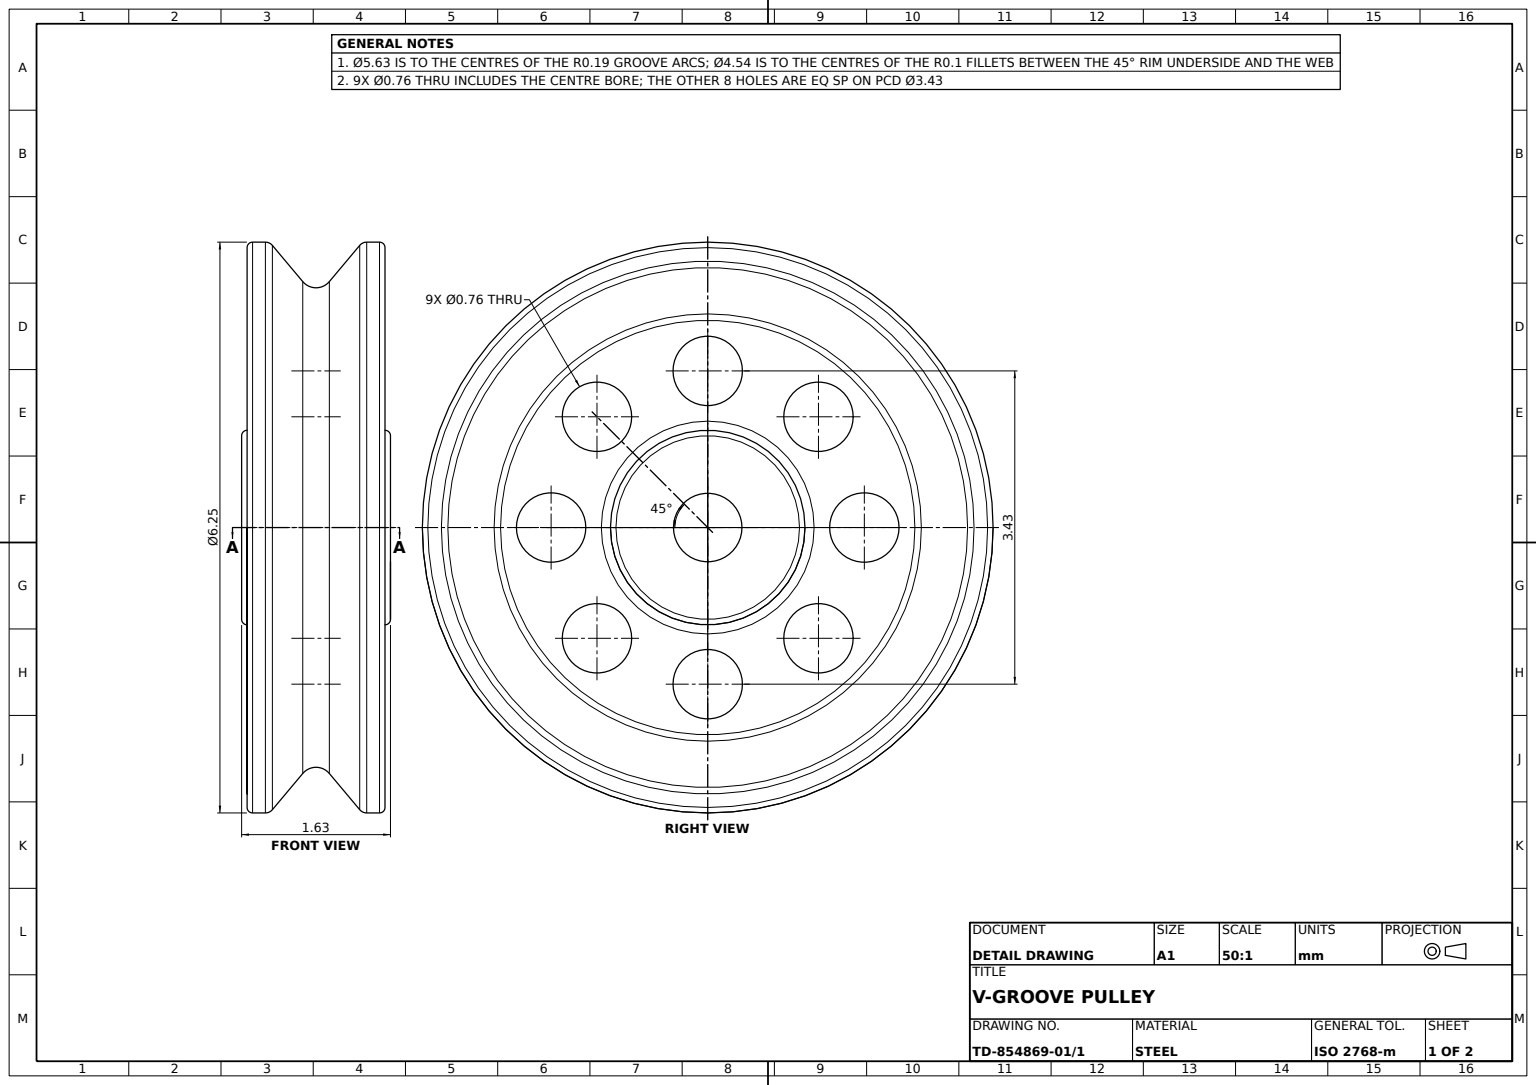
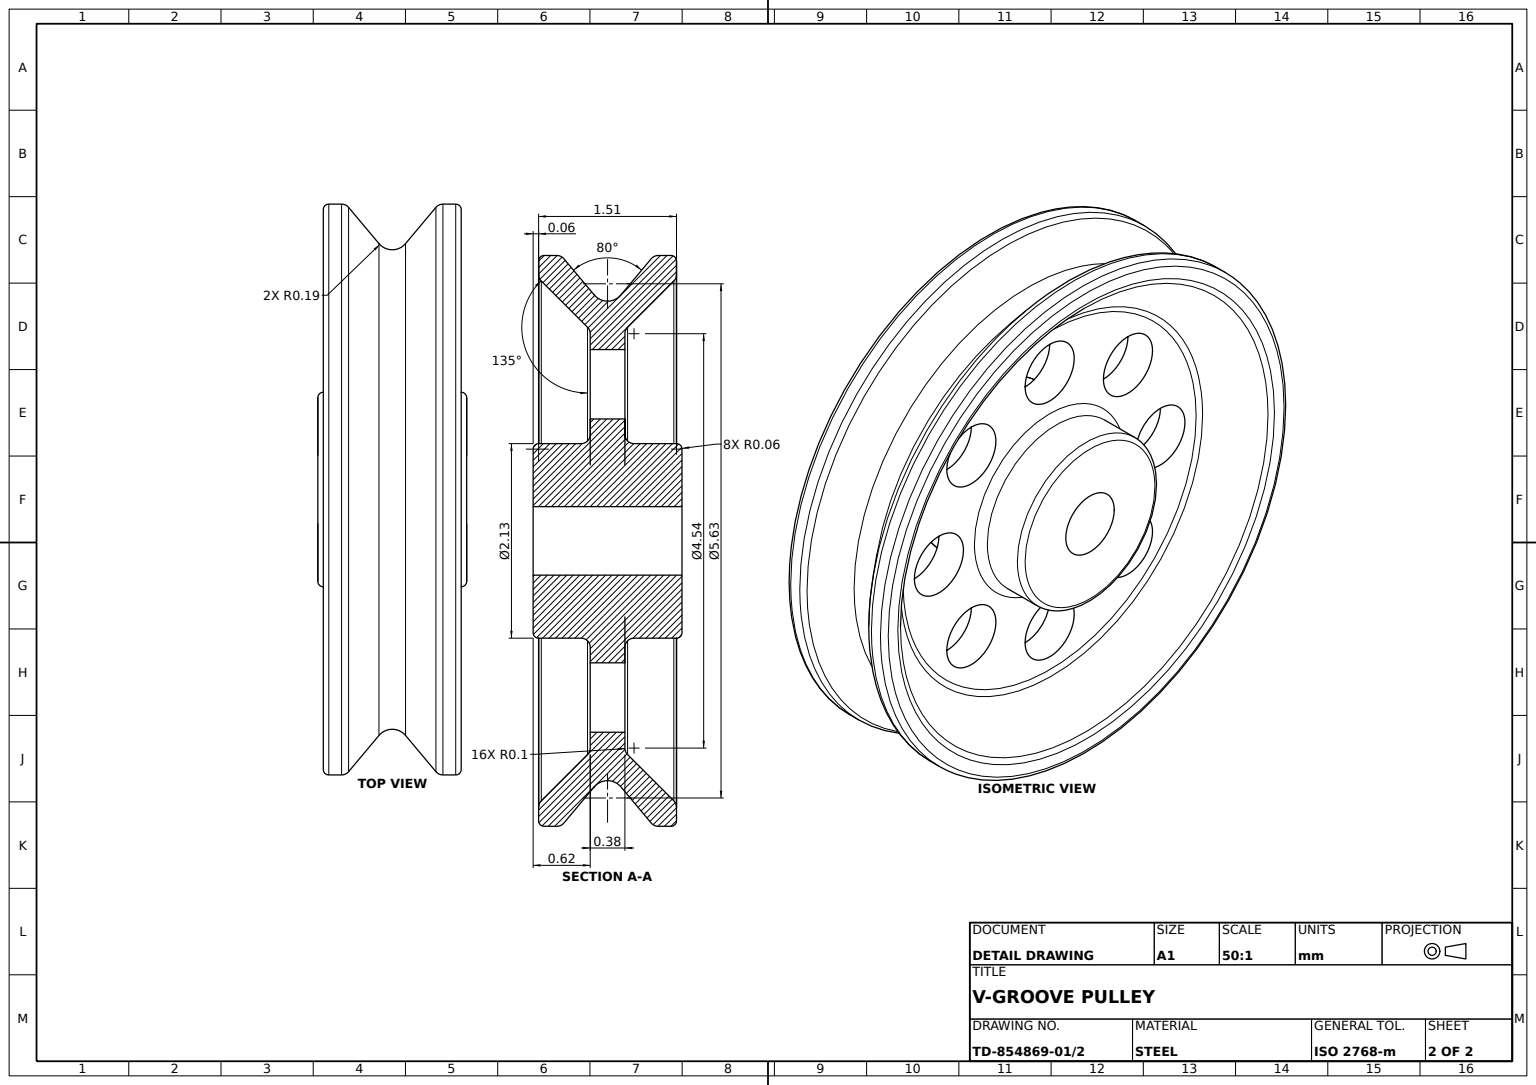
SolidWorks part; units mm, degrees
material "Plain Carbon Steel"
ref_plane "Front Plane" through (0, 0, 0) normal (0, 0, 1) x (1, 0, 0)
ref_plane "Top Plane" through (0, 0, 0) normal (0, 1, 0) x (1, 0, 0)
ref_plane "Right Plane" through (0, 0, 0) normal (1, 0, 0) x (0, 0, -1)
sketch "Pulley Profile Sketch" plane through (0, 0, 0) normal (1, 0, 0) x (0, 0, -1)
  line L0 (-29.196, 0) -> (1430.6033, 0) construction
  line L1 (0, -29.196) -> (0, 1430.6033) construction
  line L2 (0.815, 0.375) -> (-0.815, 0.375)
  line L3 (-0.815, 0.375) -> (-0.815, 1.005)
  line L4 (-0.755, 1.065) -> (-0.29, 1.065)
  line L5 (-0.19, 1.165) -> (-0.19, 2.2686)
  line L6 (-0.2193, 2.3393) -> (-0.7257, 2.8457)
  line L7 (-0.755, 2.9164) -> (-0.755, 3.065)
  line L8 (-0.695, 3.125) -> (-0.5548, 3.125)
  line L9 (-0.4782, 3.0893) -> (-0.1455, 2.6929)
  line L10 (0.1455, 2.6929) -> (0.4782, 3.0893)
  line L11 (0.5548, 3.125) -> (0.695, 3.125)
  line L12 (0.755, 3.065) -> (0.755, 2.9164)
  line L13 (0.7257, 2.8457) -> (0.2193, 2.3393)
  line L14 (0.19, 2.2686) -> (0.19, 1.165)
  line L15 (0.29, 1.065) -> (0.755, 1.065)
  line L16 (0.815, 1.005) -> (0.815, 0.375)
  arc A0 (-0.1455, 2.6929) -> (0.1455, 2.6929) centre (0, 2.815) ccw
  arc A1 (-0.755, 2.9164) -> (-0.7257, 2.8457) centre (-0.655, 2.9164) ccw
  arc A2 (0.755, 2.9164) -> (0.7257, 2.8457) centre (0.655, 2.9164) cw
  arc A3 (0.5548, 3.125) -> (0.4782, 3.0893) centre (0.5548, 3.025) ccw
  arc A4 (-0.4782, 3.0893) -> (-0.5548, 3.125) centre (-0.5548, 3.025) ccw
  arc A5 (-0.695, 3.125) -> (-0.755, 3.065) centre (-0.695, 3.065) ccw
  arc A6 (0.695, 3.125) -> (0.755, 3.065) centre (0.695, 3.065) cw
  arc A7 (0.755, 1.065) -> (0.815, 1.005) centre (0.755, 1.005) cw
  arc A8 (-0.815, 1.005) -> (-0.755, 1.065) centre (-0.755, 1.005) cw
  arc A9 (-0.2193, 2.3393) -> (-0.19, 2.2686) centre (-0.29, 2.2686) cw
  arc A10 (0.19, 2.2686) -> (0.2193, 2.3393) centre (0.29, 2.2686) cw
  arc A11 (0.19, 1.165) -> (0.29, 1.065) centre (0.29, 1.165) ccw
  arc A12 (-0.29, 1.065) -> (-0.19, 1.165) centre (-0.29, 1.165) ccw
  point P16 (0, 2.625)
  point P23 (0, 0.375)
  point P32 (-0.755, 2.875)
  point P35 (0.755, 2.875)
  point P42 (-0.755, 3.125)
  point P45 (0.755, 3.125)
  dimension "D18" = 0.1
  dimension "D19" = 0.1
  dimension "D20" = 0.1
  dimension "D21" = 0.06
  dimension "D22" = 0.06
  dimension "D23" = 0.06
  dimension "D24" = 0.1
  dimension "D25" = 0.1
  dimension "D1" = 2.815
  dimension "D2" = 2.625
  dimension "D3" = 1.63
  dimension "D4" = 0.38
  dimension "D5" = 0.19
  dimension "D6" = 80
  dimension "D7" = 40
  dimension "D8" = 1.51
  dimension "D9" = 0.755
  dimension "D10" = 0.375
  dimension "D11" = 1.065
  dimension "D12" = 1.065
  dimension "D13" = 3.125
  dimension "D14" = 3.125
  dimension "D15" = 135
  dimension "D16" = 135
  dimension "D17" = 0.25
revolve "Pulley Body" add sketch "Pulley Profile Sketch" angle 360 about L0
sketch "Lightening Holes Sketch" plane through (0, 0, 0.19) normal (0, 0, 1) x (1, 0, 0)
  line L0 (-1000, 0) -> (49000, 0) construction
  line L1 (0, -1000) -> (0, 49000) construction
  circle A0 centre (0, 0) radius 1.715 construction
  circle A1 centre (0, 1.715) radius 0.38
  circle A2 centre (-1.2127, 1.2127) radius 0.38
  circle A3 centre (-1.715, 0) radius 0.38
  circle A4 centre (-1.2127, -1.2127) radius 0.38
  circle A5 centre (0, -1.715) radius 0.38
  circle A6 centre (1.2127, -1.2127) radius 0.38
  circle A7 centre (1.715, 0) radius 0.38
  circle A8 centre (1.2127, 1.2127) radius 0.38
  point P26 (0, 0)
  dimension "D1" = 3.43
  dimension "D2" = 0.76
  dimension "D3" = 8
extrude "Lightening Holes 8xØ0.76" cut sketch "Lightening Holes Sketch" against normal through all
